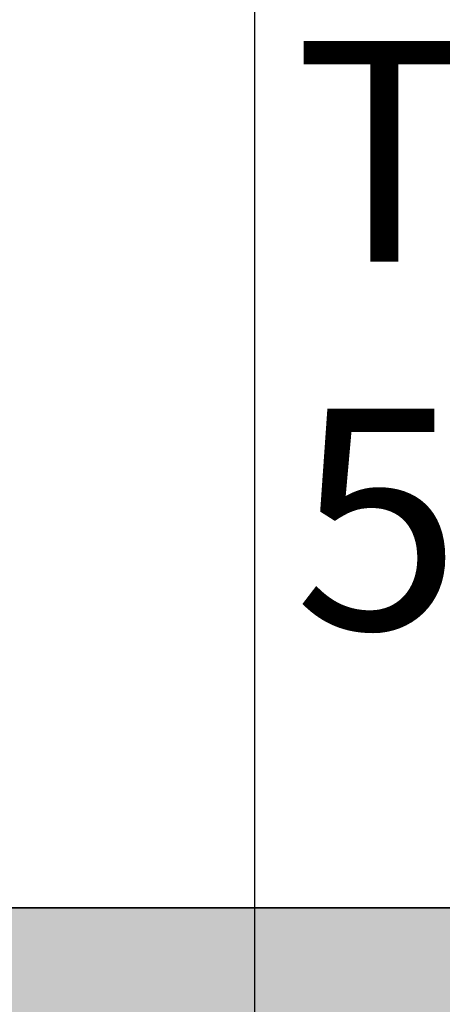
# Model space of a CAD drawing. Units: inches. Extents: x 2696 to 3240, y 1564 to 2310.
# Tile 67 of 76: x 3127 to 3144, y 2071 to 2111. Entities that reach past the tile are written whole.
import ezdxf

# ---------------------------------------------------------------- set-up
doc = ezdxf.new("R2010")
doc.units = ezdxf.units.IN
for name, color, linetype, lineweight in [('A-ANNO-DIMS', 3, 'Continuous', 18), ('A-AREA-IDEN', 7, 'Continuous', 18), ('A-WALL', 7, 'Continuous', 35), ('A-WALL-PATT', 9, 'Continuous', 13)]:
    doc.layers.add(name, color=color, linetype=linetype, lineweight=lineweight)
doc.styles.add('TIMES NEW', font='times.ttf')
doc.styles.add('YQ_DIM', font='SUPEROS.SHX', dxfattribs={"width": 0.8, "bigfont": 'HZDX.SHX'})
doc.dimstyles.new('Siddhuu', dxfattribs={"dimtxt": 6, "dimasz": 2.5, "dimexe": 1.25, "dimexo": 0.625, "dimtad": 1, "dimdec": 1, "dimlunit": 4, "dimtxsty": 'TIMES NEW', "dimcen": 2.5, "dimclrd": 256, "dimclre": 1, "dimclrt": 7, "dimadec": 0, "dimazin": 0, "dimtfac": 1, "dimtdec": 1, "dimtmove": 0, "dimatfit": 3, "dimfxl": 1, "dimtolj": 1, "dimlwd": -1, "dimarcsym": 0})

# ---------------------------------------------------------------- blocks, each defined once
blk = doc.blocks.new('*D54')
at = {"layer": 'A-ANNO-DIMS', "color": 1, "lineweight": -2, "transparency": 16777216}
for p, q in [((3124.611, 1893.826), (3124.611, 2298.451)), ((3136.611, 1893.826), (3136.611, 2298.451))]:
    blk.add_line(p, q, dxfattribs=at)
at = {"layer": 'A-ANNO-DIMS', "transparency": 16777216}
for p, q in [((3127.111, 2297.201), (3134.111, 2297.201)), ((3136.611, 2297.201), (3155.757, 2297.201))]:
    blk.add_line(p, q, dxfattribs=at)
for points in [[(3127.111, 2297.618), (3127.111, 2296.784), (3124.611, 2297.201)], [(3134.111, 2297.618), (3134.111, 2296.784), (3136.611, 2297.201)]]:
    blk.add_solid(points, dxfattribs=at)
at = {"layer": 'Defpoints', "color": 0, "transparency": 16777216}
for p in [(3136.611, 2297.201), (3124.611, 1893.201), (3136.611, 1893.201)]:
    blk.add_point(p, dxfattribs=at)
at = {"layer": 'A-ANNO-DIMS', "color": 7, "transparency": 16777216, "insert": (3147.434, 2300.878), "char_height": 6, "attachment_point": 5, "style": 'TIMES NEW'}
blk.add_mtext('\\A1;1\'-0"', dxfattribs=at)

msp = doc.modelspace()

# ---------------------------------------------------------------- hatches: boundary and pattern name
at = {"layer": 'A-WALL-PATT', "transparency": 33554556}
h = msp.add_hatch(color=256, dxfattribs=at)
h.dxf.hatch_style = 1
h.paths.add_polyline_path([(2879.111, 2253.201), (2905.91, 2253.201), (2905.91, 2262.201), (2841.889, 2262.201), (2841.889, 2253.201), (2870.111, 2253.201), (2870.111, 2176.601), (2965.709, 2176.601), (2965.709, 2206.701), (2973.583, 2206.701), (2973.583, 2215.701), (2965.709, 2215.701), (2965.709, 2262.201), (2929.91, 2262.201), (2929.91, 2253.201), (2956.709, 2253.201), (2956.709, 2185.601), (2879.111, 2185.601)])
h.paths.add_polyline_path([(2782.834, 2262.201), (2745.611, 2262.201), (2745.611, 2228.729), (2754.611, 2228.729), (2754.611, 2253.201), (2782.834, 2253.201)])
h.paths.add_polyline_path([(2754.611, 2136.201), (2965.709, 2136.201), (2965.709, 2145.201), (2879.111, 2145.201), (2879.111, 2147.074), (2877.34, 2147.074), (2870.111, 2147.074), (2870.111, 2145.201), (2754.611, 2145.201), (2754.611, 2169.674), (2745.611, 2169.674), (2745.611, 2000.201), (2754.611, 2000.201), (2754.611, 2019.201), (2849.083, 2019.201), (2849.083, 2023.701), (2841.209, 2023.701), (2841.209, 2051.827), (2836.709, 2051.827), (2836.709, 2023.701), (2754.611, 2023.701), (2754.611, 2091.201), (2836.709, 2091.201), (2836.709, 2087.827), (2841.209, 2087.827), (2841.209, 2095.701), (2754.611, 2095.701)])
h.paths.add_polyline_path([(2965.709, 2136.201), (2956.709, 2136.201), (2956.709, 2023.701), (2885.083, 2023.701), (2885.083, 2019.201), (2956.709, 2019.201), (2956.709, 1950.575), (2965.709, 1950.575), (2965.709, 1980.201), (2973.583, 1980.201), (2973.583, 1989.201), (2965.709, 1989.201)])
h.paths.add_polyline_path([(2754.611, 1906.701), (2880.209, 1906.701), (2884.709, 1906.701), (2956.709, 1906.701), (2956.709, 1792.701), (2944.709, 1792.701), (2944.709, 1783.701), (2956.709, 1783.701), (2956.709, 1740.201), (2884.709, 1740.201), (2884.709, 1783.701), (2896.709, 1783.701), (2896.709, 1792.701), (2884.709, 1792.701), (2884.709, 1846.701), (2880.209, 1846.701), (2880.209, 1740.201), (2754.611, 1740.201), (2754.611, 1777.201), (2745.611, 1777.201), (2745.611, 1692.701), (2754.611, 1692.701), (2754.611, 1731.201), (2956.709, 1731.201), (2956.709, 1723.327), (2965.709, 1723.327), (2965.709, 1884.201), (2973.583, 1884.201), (2973.583, 1893.201), (2965.709, 1893.201), (2965.709, 1914.575), (2956.709, 1914.575), (2956.709, 1911.201), (2754.611, 1911.201), (2754.611, 1930.201), (2745.611, 1930.201), (2745.611, 1817.201), (2754.611, 1817.201), (2754.611, 1854.201), (2826.611, 1854.201), (2826.611, 1868.827), (2822.111, 1868.827), (2822.111, 1858.701), (2754.611, 1858.701)])
h.paths.add_polyline_path([(2965.709, 1656.201), (3008.237, 1656.201), (3008.237, 1665.201), (2965.709, 1665.201), (2965.709, 1693.327), (2956.709, 1693.327), (2956.709, 1686.201), (2934.583, 1686.201), (2934.583, 1681.701), (2956.709, 1681.701), (2956.709, 1614.201), (2896.709, 1614.201), (2896.709, 1681.701), (2904.583, 1681.701), (2904.583, 1686.201), (2892.209, 1686.201), (2892.209, 1614.201), (2858.41, 1614.201), (2858.41, 1605.201), (2965.709, 1605.201)])
h.paths.add_polyline_path([(2788.41, 1614.201), (2754.611, 1614.201), (2754.611, 1652.701), (2745.611, 1652.701), (2745.611, 1605.201), (2788.41, 1605.201)])
h.paths.add_polyline_path([(3199.611, 1633.048), (3190.611, 1633.048), (3190.611, 1614.201), (3082.611, 1614.201), (3082.611, 1665.201), (3070.237, 1665.201), (3070.237, 1656.201), (3078.111, 1656.201), (3078.111, 1605.201), (3199.611, 1605.201)])
h.paths.add_polyline_path([(3199.611, 1702.048), (3190.611, 1702.048), (3190.611, 1699.701), (3106.611, 1699.701), (3106.611, 1747.701), (3190.611, 1747.701), (3190.611, 1752.201), (3082.611, 1752.201), (3082.611, 1760.075), (3078.111, 1760.075), (3078.111, 1747.701), (3102.111, 1747.701), (3102.111, 1699.701), (3078.111, 1699.701), (3078.111, 1695.201), (3190.611, 1695.201), (3190.611, 1676.355), (3199.611, 1676.355)])
h.paths.add_polyline_path([(3199.611, 1783.201), (3190.611, 1783.201), (3190.611, 1745.355), (3199.611, 1745.355)])
h.paths.add_polyline_path([(3082.611, 1884.201), (3190.611, 1884.201), (3190.611, 1853.201), (3199.611, 1853.201), (3199.611, 1901.701), (3190.611, 1901.701), (3190.611, 1893.201), (3005.583, 1893.201), (3005.583, 1891.281), (3005.583, 1884.201), (3078.111, 1884.201), (3078.111, 1792.075), (3082.611, 1792.075)])
h.paths.add_polyline_path([(3199.611, 1994.701), (3190.611, 1994.701), (3190.611, 1989.201), (3073.709, 1989.201), (3073.709, 2034.201), (3069.209, 2034.201), (3069.209, 1989.201), (3005.583, 1989.201), (3005.583, 1980.201), (3190.611, 1980.201), (3190.611, 1971.701), (3199.611, 1971.701)])
h.paths.add_polyline_path([(3199.611, 2155.201), (3190.611, 2155.201), (3190.611, 2064.701), (3199.611, 2064.701)])
h.paths.add_polyline_path([(3190.611, 2074.701), (3106.611, 2074.701), (3106.611, 2122.701), (3190.611, 2122.701), (3190.611, 2127.201), (3082.709, 2127.201), (3082.709, 2135.075), (3073.709, 2135.075), (3073.709, 2122.701), (3102.111, 2122.701), (3102.111, 2074.701), (3069.209, 2074.701), (3069.209, 2070.201), (3190.611, 2070.201)])
h.paths.add_polyline_path([(3082.709, 2253.201), (3190.611, 2253.201), (3190.611, 2225.201), (3199.611, 2225.201), (3199.611, 2262.201), (3073.709, 2262.201), (3073.709, 2215.701), (3035.583, 2215.701), (3035.583, 2206.701), (3073.709, 2206.701), (3073.709, 2171.075), (3082.709, 2171.075)])

# ---------------------------------------------------------------- linework, layer by layer
at = {"layer": 'A-WALL'}
msp.add_line((3106.611, 2074.701), (3190.611, 2074.701), dxfattribs=at)

# ---------------------------------------------------------------- texts
at = {"layer": 'A-AREA-IDEN', "insert": (3138.221, 2110.067), "char_height": 9, "attachment_point": 1, "style": 'YQ_DIM'}
msp.add_mtext_dynamic_manual_height_columns('TOILET\\P5\'X5\'4.5"', width=48.00324, gutter_width=12.5, heights=[0], dxfattribs=at)

# ---------------------------------------------------------------- dimensions: what is measured, and where the dimension line sits
at = {"layer": 'A-ANNO-DIMS'}
dim = msp.add_linear_dim(base=(3136.611, 2297.201), p1=(3124.611, 1893.201), p2=(3136.611, 1893.201), dimstyle='Siddhuu', override={"dimdec": 1, "dimlfac": 1, "dimrnd": 0, "dimzin": 1, "dimdsep": 46, "dimlunit": 4, "dimfrac": 2}, dxfattribs=at)
dim.commit()
dim.dimension.update_dxf_attribs({"geometry": '*D54', "text_midpoint": (3147.434, 2300.878)})

doc.saveas('drawing.dxf')
